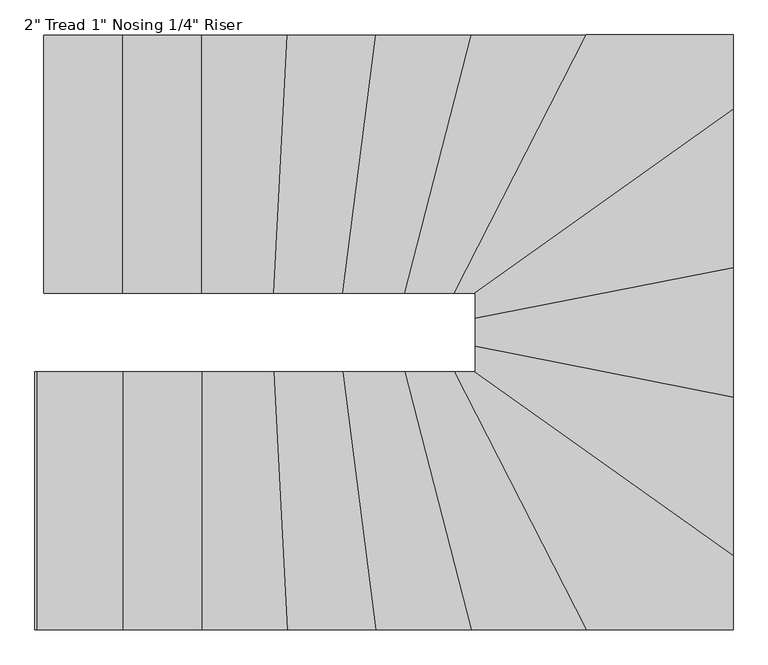
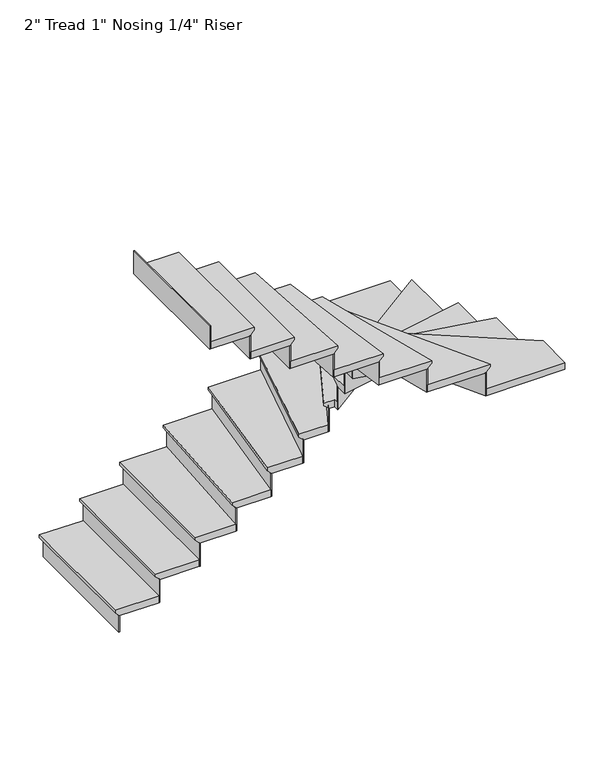
"""IFC4 building model written with IfcOpenShell, lengths in millimetres: stair flight geometry."""

from ifc_helpers import new_model, si_unit, origin, place, context, project, spatial, faceted_brep, source, transform, mapped, element, save


def stair_flight_2bffc1af(model_context):
    return source(origin(), model_context, "Body", "Brep", [
        faceted_brep([(-6984.582258, 1695.3645941, 150.2833333), (-6984.582258, 1695.3645941, 169.3333333), (-6984.582258, 2609.7645941, 169.3333333), (-6984.582258, 2609.7645941, 150.2833333), (-6959.182258, 1695.3645941, 124.8833333), (-6959.182258, 2609.7645941, 124.8833333), (-6679.782258, 1695.3645941, 169.3333333), (-6679.782258, 2609.7645941, 169.3333333), (-6959.182258, 2609.7645941, 118.5333333), (-6679.782258, 2609.7645941, 118.5333333), (-6679.782258, 1695.3645941, 118.5333333), (-6959.182258, 1695.3645941, 118.5333333)], [[[0, 1, 2, 3]], [[4, 0, 3, 5]], [[2, 1, 6, 7]], [[8, 9, 10, 11]], [[2, 7, 9, 8, 5, 3]], [[8, 11, 4, 5]], [[6, 1, 0, 4, 11, 10]], [[7, 6, 10, 9]]]),
        faceted_brep([(-6959.182258, 1695.3645941, 118.5333333), (-6959.182258, 1695.3645941, 0.0), (-6952.832258, 1695.3645941, 0.0), (-6952.832258, 1695.3645941, 118.5333333), (-6959.182258, 2609.7645941, 118.5333333), (-6952.832258, 2609.7645941, 118.5333333), (-6952.832258, 2609.7645941, 0.0), (-6959.182258, 2609.7645941, 0.0)], [[[0, 1, 2, 3]], [[4, 5, 6, 7]], [[1, 0, 4, 7]], [[2, 1, 7, 6]], [[3, 2, 6, 5]], [[0, 3, 5, 4]]]),
        faceted_brep([(-6679.782258, 1695.3645941, 287.8666667), (-6679.782258, 1695.3645941, 118.5333333), (-6673.432258, 1695.3645941, 118.5333333), (-6673.432258, 1695.3645941, 287.8666667), (-6679.782258, 2609.7645941, 287.8666667), (-6673.432258, 2609.7645941, 287.8666667), (-6673.432258, 2609.7645941, 118.5333333), (-6679.782258, 2609.7645941, 118.5333333)], [[[0, 1, 2, 3]], [[4, 5, 6, 7]], [[1, 0, 4, 7]], [[2, 1, 7, 6]], [[3, 2, 6, 5]], [[0, 3, 5, 4]]]),
        faceted_brep([(-6705.182258, 2609.7645941, 338.6666667), (-6705.182258, 1695.3645941, 338.6666667), (-6400.382258, 1695.3645941, 338.6666667), (-6400.382258, 2609.7645941, 338.6666667), (-6679.782258, 2609.7645941, 287.8666667), (-6400.382258, 2609.7645941, 287.8666667), (-6400.382258, 1695.3645941, 287.8666667), (-6679.782258, 1695.3645941, 287.8666667), (-6679.782258, 2609.7645941, 294.2166667), (-6705.182258, 2609.7645941, 319.6166667), (-6679.782258, 1695.3645941, 294.2166667), (-6705.182258, 1695.3645941, 319.6166667)], [[[0, 1, 2, 3]], [[4, 5, 6, 7]], [[0, 3, 5, 4, 8, 9]], [[4, 7, 10, 8]], [[2, 1, 11, 10, 7, 6]], [[3, 2, 6, 5]], [[11, 1, 0, 9]], [[10, 11, 9, 8]]]),
        faceted_brep([(-6400.382258, 1695.3645941, 457.2), (-6400.382258, 1695.3645941, 287.8666667), (-6394.032258, 1695.3645941, 287.8666667), (-6394.032258, 1695.3645941, 457.2), (-6400.382258, 2609.7645941, 457.2), (-6394.032258, 2609.7645941, 457.2), (-6394.032258, 2609.7645941, 287.8666667), (-6400.382258, 2609.7645941, 287.8666667)], [[[0, 1, 2, 3]], [[4, 5, 6, 7]], [[1, 0, 4, 7]], [[2, 1, 7, 6]], [[3, 2, 6, 5]], [[0, 3, 5, 4]]]),
        faceted_brep([(-6425.782258, 2609.7645941, 508.0), (-6425.782258, 1695.3645941, 508.0), (-6144.7150966, 1695.3645941, 508.0), (-6097.1808262, 2609.7645941, 508.0), (-6400.382258, 2609.7645941, 457.2), (-6097.1808262, 2609.7645941, 457.2), (-6144.7150966, 1695.3645941, 457.2), (-6400.382258, 1695.3645941, 457.2), (-6400.382258, 2609.7645941, 463.55), (-6425.782258, 2609.7645941, 488.95), (-6400.382258, 1695.3645941, 463.55), (-6425.782258, 1695.3645941, 488.95)], [[[0, 1, 2, 3]], [[4, 5, 6, 7]], [[0, 3, 5, 4, 8, 9]], [[4, 7, 10, 8]], [[2, 1, 11, 10, 7, 6]], [[3, 2, 6, 5]], [[11, 1, 0, 9]], [[10, 11, 9, 8]]]),
        faceted_brep([(-6144.7150966, 1695.3645941, 626.5333333), (-6144.7150966, 1695.3645941, 457.2), (-6138.3565224, 1695.3645941, 457.2), (-6138.3565224, 1695.3645941, 626.5333333), (-6097.1808262, 2609.7645941, 626.5333333), (-6090.822252, 2609.7645941, 626.5333333), (-6090.822252, 2609.7645941, 457.2), (-6097.1808262, 2609.7645941, 457.2)], [[[0, 1, 2, 3]], [[4, 5, 6, 7]], [[1, 0, 4, 7]], [[2, 1, 7, 6]], [[3, 2, 6, 5]], [[0, 3, 5, 4]]]),
        faceted_brep([(-6122.6151228, 2609.7645941, 677.3333333), (-6170.1493932, 1695.3645941, 677.3333333), (-5900.5483967, 1695.3645941, 677.3333333), (-5782.1923451, 2609.7645941, 677.3333333), (-6097.1808262, 2609.7645941, 626.5333333), (-5782.1923451, 2609.7645941, 626.5333333), (-5900.5483967, 1695.3645941, 626.5333333), (-6144.7150966, 1695.3645941, 626.5333333), (-6097.1808262, 2609.7645941, 632.8833333), (-6122.6151228, 2609.7645941, 658.2833333), (-6144.7150966, 1695.3645941, 632.8833333), (-6170.1493932, 1695.3645941, 658.2833333)], [[[0, 1, 2, 3]], [[4, 5, 6, 7]], [[0, 3, 5, 4, 8, 9]], [[4, 7, 10, 8]], [[2, 1, 11, 10, 7, 6]], [[3, 2, 6, 5]], [[11, 1, 0, 9]], [[10, 11, 9, 8]]]),
        faceted_brep([(-5900.5483967, 1695.3645941, 795.8666667), (-5900.5483967, 1695.3645941, 626.5333333), (-5894.145425, 1695.3645941, 626.5333333), (-5894.145425, 1695.3645941, 795.8666667), (-5782.1923451, 2609.7645941, 795.8666667), (-5775.7893733, 2609.7645941, 795.8666667), (-5775.7893733, 2609.7645941, 626.5333333), (-5782.1923451, 2609.7645941, 626.5333333)], [[[0, 1, 2, 3]], [[4, 5, 6, 7]], [[1, 0, 4, 7]], [[2, 1, 7, 6]], [[3, 2, 6, 5]], [[0, 3, 5, 4]]]),
        faceted_brep([(-5807.8042322, 2609.7645941, 846.6666667), (-5926.1602839, 1695.3645941, 846.6666667), (-5678.9211743, 1695.3645941, 846.6666667), (-5443.7907269, 2609.7645941, 846.6666667), (-5782.1923451, 2609.7645941, 795.8666667), (-5443.7907269, 2609.7645941, 795.8666667), (-5678.9211743, 1695.3645941, 795.8666667), (-5900.5483967, 1695.3645941, 795.8666667), (-5782.1923451, 2609.7645941, 802.2166667), (-5807.8042322, 2609.7645941, 827.6166667), (-5900.5483967, 1695.3645941, 802.2166667), (-5926.1602839, 1695.3645941, 827.6166667)], [[[0, 1, 2, 3]], [[4, 5, 6, 7]], [[0, 3, 5, 4, 8, 9]], [[4, 7, 10, 8]], [[2, 1, 11, 10, 7, 6]], [[3, 2, 6, 5]], [[11, 1, 0, 9]], [[10, 11, 9, 8]]]),
        faceted_brep([(-5678.9211743, 1695.3645941, 965.2), (-5678.9211743, 1695.3645941, 795.8666667), (-5672.3645974, 1695.3645941, 795.8666667), (-5672.3645974, 1695.3645941, 965.2), (-5443.7907269, 2609.7645941, 965.2), (-5437.23415, 2609.7645941, 965.2), (-5437.23415, 2609.7645941, 795.8666667), (-5443.7907269, 2609.7645941, 795.8666667)], [[[0, 1, 2, 3]], [[4, 5, 6, 7]], [[1, 0, 4, 7]], [[2, 1, 7, 6]], [[3, 2, 6, 5]], [[0, 3, 5, 4]]]),
        faceted_brep([(-5470.0170343, 2609.7645941, 1016.0), (-5705.1474817, 1695.3645941, 1016.0), (-5502.5745382, 1695.3645941, 1016.0), (-5033.7499169, 2609.7645941, 1016.0), (-5443.7907269, 2609.7645941, 965.2), (-5033.7499169, 2609.7645941, 965.2), (-5502.5745382, 1695.3645941, 965.2), (-5678.9211743, 1695.3645941, 965.2), (-5443.7907269, 2609.7645941, 971.55), (-5470.0170343, 2609.7645941, 996.95), (-5678.9211743, 1695.3645941, 971.55), (-5705.1474817, 1695.3645941, 996.95)], [[[0, 1, 2, 3]], [[4, 5, 6, 7]], [[0, 3, 5, 4, 8, 9]], [[4, 7, 10, 8]], [[2, 1, 11, 10, 7, 6]], [[3, 2, 6, 5]], [[11, 1, 0, 9]], [[10, 11, 9, 8]]]),
        faceted_brep([(-5502.5745382, 1695.3645941, 1134.5333333), (-5502.5745382, 1695.3645941, 965.2), (-5495.4385551, 1695.3645941, 965.2), (-5495.4385551, 1695.3645941, 1134.5333333), (-5033.7499169, 2609.7645941, 1134.5333333), (-5026.6139337, 2609.7645941, 1134.5333333), (-5026.6139337, 2609.7645941, 965.2), (-5033.7499169, 2609.7645941, 965.2)], [[[0, 1, 2, 3]], [[4, 5, 6, 7]], [[1, 0, 4, 7]], [[2, 1, 7, 6]], [[3, 2, 6, 5]], [[0, 3, 5, 4]]]),
        faceted_brep([(-4542.4505662, 2316.0834604, 1185.3333333), (-4542.4505662, 2609.7645941, 1185.3333333), (-5062.2938494, 2609.7645941, 1185.3333333), (-5531.1184707, 1695.3645941, 1185.3333333), (-5456.8505662, 1695.3645941, 1185.3333333), (-5456.8505662, 1665.8095113, 1185.3333333), (-4542.4505662, 2609.7645941, 1134.5333333), (-4542.4505662, 2316.0834604, 1134.5333333), (-5456.8505662, 1665.8095113, 1134.5333333), (-5456.8505662, 1695.3645941, 1134.5333333), (-5502.5745382, 1695.3645941, 1134.5333333), (-5033.7499169, 2609.7645941, 1134.5333333), (-5033.7499169, 2609.7645941, 1140.8833333), (-5062.2938494, 2609.7645941, 1166.2833333), (-5502.5745382, 1695.3645941, 1140.8833333), (-5531.1184707, 1695.3645941, 1166.2833333)], [[[0, 1, 2, 3, 4, 5]], [[6, 7, 8, 9, 10, 11]], [[1, 0, 7, 6]], [[2, 1, 6, 11, 12, 13]], [[11, 10, 14, 12]], [[4, 3, 15, 14, 10, 9]], [[5, 4, 9, 8]], [[0, 5, 8, 7]], [[15, 3, 2, 13]], [[14, 15, 13, 12]]]),
        faceted_brep([(-5456.8505662, 1665.8095113, 1303.8666667), (-5456.8505662, 1665.8095113, 1134.5333333), (-5456.8505662, 1658.0175365, 1134.5333333), (-5456.8505662, 1658.0175365, 1303.8666667), (-4542.4505662, 2316.0834604, 1303.8666667), (-4542.4505662, 2308.2914857, 1303.8666667), (-4542.4505662, 2308.2914857, 1134.5333333), (-4542.4505662, 2316.0834604, 1134.5333333)], [[[0, 1, 2, 3]], [[4, 5, 6, 7]], [[1, 0, 4, 7]], [[2, 1, 7, 6]], [[3, 2, 6, 5]], [[0, 3, 5, 4]]]),
        faceted_brep([(-4542.4505662, 2347.2513596, 1354.6666667), (-5456.8505662, 1696.9774105, 1354.6666667), (-5456.8505662, 1579.3554242, 1354.6666667), (-4542.4505662, 1759.5962806, 1354.6666667), (-4542.4505662, 2316.0834604, 1303.8666667), (-4542.4505662, 1759.5962806, 1303.8666667), (-5456.8505662, 1579.3554242, 1303.8666667), (-5456.8505662, 1665.8095113, 1303.8666667), (-4542.4505662, 2316.0834604, 1310.2166667), (-4542.4505662, 2347.2513596, 1335.6166667), (-5456.8505662, 1665.8095113, 1310.2166667), (-5456.8505662, 1696.9774105, 1335.6166667)], [[[0, 1, 2, 3]], [[4, 5, 6, 7]], [[0, 3, 5, 4, 8, 9]], [[4, 7, 10, 8]], [[2, 1, 11, 10, 7, 6]], [[3, 2, 6, 5]], [[11, 1, 0, 9]], [[10, 11, 9, 8]]]),
        faceted_brep([(-5456.8505662, 1579.3554242, 1473.2), (-5456.8505662, 1579.3554242, 1303.8666667), (-5456.8505662, 1572.8832388, 1303.8666667), (-5456.8505662, 1572.8832388, 1473.2), (-4542.4505662, 1759.5962806, 1473.2), (-4542.4505662, 1753.1240951, 1473.2), (-4542.4505662, 1753.1240951, 1303.8666667), (-4542.4505662, 1759.5962806, 1303.8666667)], [[[0, 1, 2, 3]], [[4, 5, 6, 7]], [[1, 0, 4, 7]], [[2, 1, 7, 6]], [[3, 2, 6, 5]], [[0, 3, 5, 4]]]),
        faceted_brep([(-4542.4505662, 1785.4850223, 1524.0), (-5456.8505662, 1605.244166, 1524.0), (-5456.8505662, 1480.1962806, 1524.0), (-4542.4505662, 1299.9554242, 1524.0), (-4542.4505662, 1759.5962806, 1473.2), (-4542.4505662, 1299.9554242, 1473.2), (-5456.8505662, 1480.1962806, 1473.2), (-5456.8505662, 1579.3554242, 1473.2), (-4542.4505662, 1759.5962806, 1479.55), (-4542.4505662, 1785.4850223, 1504.95), (-5456.8505662, 1579.3554242, 1479.55), (-5456.8505662, 1605.244166, 1504.95)], [[[0, 1, 2, 3]], [[4, 5, 6, 7]], [[0, 3, 5, 4, 8, 9]], [[4, 7, 10, 8]], [[2, 1, 11, 10, 7, 6]], [[3, 2, 6, 5]], [[11, 1, 0, 9]], [[10, 11, 9, 8]]]),
        faceted_brep([(-5456.8505662, 1480.1962806, 1642.5333333), (-5456.8505662, 1480.1962806, 1473.2), (-5456.8505662, 1473.7240951, 1473.2), (-5456.8505662, 1473.7240951, 1642.5333333), (-4542.4505662, 1299.9554242, 1642.5333333), (-4542.4505662, 1293.4832388, 1642.5333333), (-4542.4505662, 1293.4832388, 1473.2), (-4542.4505662, 1299.9554242, 1473.2)], [[[0, 1, 2, 3]], [[4, 5, 6, 7]], [[1, 0, 4, 7]], [[2, 1, 7, 6]], [[3, 2, 6, 5]], [[0, 3, 5, 4]]]),
        faceted_brep([(-4542.4505662, 1325.844166, 1693.3333333), (-5456.8505662, 1506.0850223, 1693.3333333), (-5456.8505662, 1415.9645941, 1693.3333333), (-5502.9460407, 1415.9645941, 1693.3333333), (-4542.4505662, 732.9099295, 1693.3333333), (-4542.4505662, 1299.9554242, 1642.5333333), (-4542.4505662, 732.9099295, 1642.5333333), (-5502.9460407, 1415.9645941, 1642.5333333), (-5456.8505662, 1415.9645941, 1642.5333333), (-5456.8505662, 1480.1962806, 1642.5333333), (-4542.4505662, 1299.9554242, 1648.8833333), (-4542.4505662, 1325.844166, 1674.2833333), (-5456.8505662, 1480.1962806, 1648.8833333), (-5456.8505662, 1506.0850223, 1674.2833333)], [[[0, 1, 2, 3, 4]], [[5, 6, 7, 8, 9]], [[0, 4, 6, 5, 10, 11]], [[5, 9, 12, 10]], [[2, 1, 13, 12, 9, 8]], [[3, 2, 8, 7]], [[4, 3, 7, 6]], [[13, 1, 0, 11]], [[12, 13, 11, 10]]]),
        faceted_brep([(-5502.9460407, 1415.9645941, 1811.8666667), (-5502.9460407, 1415.9645941, 1642.5333333), (-5513.9029332, 1415.9645941, 1642.5333333), (-5513.9029332, 1415.9645941, 1811.8666667), (-4542.4505662, 732.9099295, 1811.8666667), (-4542.4505662, 725.1179547, 1811.8666667), (-4542.4505662, 725.1179547, 1642.5333333), (-4542.4505662, 732.9099295, 1642.5333333)], [[[0, 1, 2, 3]], [[4, 5, 6, 7]], [[1, 0, 4, 7]], [[2, 1, 7, 6]], [[3, 2, 6, 5]], [[0, 3, 5, 4]]]),
        faceted_brep([(-5090.8377819, 501.5645941, 1862.6666667), (-4542.4505662, 501.5645941, 1862.6666667), (-4542.4505662, 764.0778287, 1862.6666667), (-5459.1184707, 1415.9645941, 1862.6666667), (-5559.6624033, 1415.9645941, 1862.6666667), (-4542.4505662, 501.5645941, 1811.8666667), (-5090.8377819, 501.5645941, 1811.8666667), (-5559.6624033, 1415.9645941, 1811.8666667), (-5502.9460407, 1415.9645941, 1811.8666667), (-4542.4505662, 732.9099295, 1811.8666667), (-4542.4505662, 732.9099295, 1818.2166667), (-4542.4505662, 764.0778287, 1843.6166667), (-5502.9460407, 1415.9645941, 1818.2166667), (-5459.1184707, 1415.9645941, 1843.6166667)], [[[0, 1, 2, 3, 4]], [[5, 6, 7, 8, 9]], [[1, 0, 6, 5]], [[2, 1, 5, 9, 10, 11]], [[9, 8, 12, 10]], [[4, 3, 13, 12, 8, 7]], [[0, 4, 7, 6]], [[13, 3, 2, 11]], [[12, 13, 11, 10]]]),
        faceted_brep([(-5559.6624033, 1415.9645941, 1981.2), (-5559.6624033, 1415.9645941, 1811.8666667), (-5566.7983864, 1415.9645941, 1811.8666667), (-5566.7983864, 1415.9645941, 1981.2), (-5090.8377819, 501.5645941, 1981.2), (-5097.9737651, 501.5645941, 1981.2), (-5097.9737651, 501.5645941, 1811.8666667), (-5090.8377819, 501.5645941, 1811.8666667)], [[[0, 1, 2, 3]], [[4, 5, 6, 7]], [[1, 0, 4, 7]], [[2, 1, 7, 6]], [[3, 2, 6, 5]], [[0, 3, 5, 4]]]),
        faceted_brep([(-5062.2938494, 501.5645941, 2032.0), (-5531.1184707, 1415.9645941, 2032.0), (-5731.3737892, 1415.9645941, 2032.0), (-5496.2433418, 501.5645941, 2032.0), (-5090.8377819, 501.5645941, 1981.2), (-5496.2433418, 501.5645941, 1981.2), (-5731.3737892, 1415.9645941, 1981.2), (-5559.6624033, 1415.9645941, 1981.2), (-5090.8377819, 501.5645941, 1987.55), (-5062.2938494, 501.5645941, 2012.95), (-5559.6624033, 1415.9645941, 1987.55), (-5531.1184707, 1415.9645941, 2012.95)], [[[0, 1, 2, 3]], [[4, 5, 6, 7]], [[0, 3, 5, 4, 8, 9]], [[4, 7, 10, 8]], [[2, 1, 11, 10, 7, 6]], [[3, 2, 6, 5]], [[11, 1, 0, 9]], [[10, 11, 9, 8]]]),
        faceted_brep([(-5731.3737892, 1415.9645941, 2150.5333333), (-5731.3737892, 1415.9645941, 1981.2), (-5737.9303661, 1415.9645941, 1981.2), (-5737.9303661, 1415.9645941, 2150.5333333), (-5496.2433418, 501.5645941, 2150.5333333), (-5502.7999187, 501.5645941, 2150.5333333), (-5502.7999187, 501.5645941, 1981.2), (-5496.2433418, 501.5645941, 1981.2)], [[[0, 1, 2, 3]], [[4, 5, 6, 7]], [[1, 0, 4, 7]], [[2, 1, 7, 6]], [[3, 2, 6, 5]], [[0, 3, 5, 4]]]),
        faceted_brep([(-5470.0170343, 501.5645941, 2201.3333333), (-5705.1474817, 1415.9645941, 2201.3333333), (-5951.772171, 1415.9645941, 2201.3333333), (-5833.4161193, 501.5645941, 2201.3333333), (-5496.2433418, 501.5645941, 2150.5333333), (-5833.4161193, 501.5645941, 2150.5333333), (-5951.772171, 1415.9645941, 2150.5333333), (-5731.3737892, 1415.9645941, 2150.5333333), (-5496.2433418, 501.5645941, 2156.8833333), (-5470.0170343, 501.5645941, 2182.2833333), (-5731.3737892, 1415.9645941, 2156.8833333), (-5705.1474817, 1415.9645941, 2182.2833333)], [[[0, 1, 2, 3]], [[4, 5, 6, 7]], [[0, 3, 5, 4, 8, 9]], [[4, 7, 10, 8]], [[2, 1, 11, 10, 7, 6]], [[3, 2, 6, 5]], [[11, 1, 0, 9]], [[10, 11, 9, 8]]]),
        faceted_brep([(-5951.772171, 1415.9645941, 2319.8666667), (-5951.772171, 1415.9645941, 2150.5333333), (-5958.1751428, 1415.9645941, 2150.5333333), (-5958.1751428, 1415.9645941, 2319.8666667), (-5833.4161193, 501.5645941, 2319.8666667), (-5839.8190911, 501.5645941, 2319.8666667), (-5839.8190911, 501.5645941, 2150.5333333), (-5833.4161193, 501.5645941, 2150.5333333)], [[[0, 1, 2, 3]], [[4, 5, 6, 7]], [[1, 0, 4, 7]], [[2, 1, 7, 6]], [[3, 2, 6, 5]], [[0, 3, 5, 4]]]),
        faceted_brep([(-5807.8042322, 501.5645941, 2370.6666667), (-5926.1602839, 1415.9645941, 2370.6666667), (-6195.5836899, 1415.9645941, 2370.6666667), (-6148.0494195, 501.5645941, 2370.6666667), (-5833.4161193, 501.5645941, 2319.8666667), (-6148.0494195, 501.5645941, 2319.8666667), (-6195.5836899, 1415.9645941, 2319.8666667), (-5951.772171, 1415.9645941, 2319.8666667), (-5833.4161193, 501.5645941, 2326.2166667), (-5807.8042322, 501.5645941, 2351.6166667), (-5951.772171, 1415.9645941, 2326.2166667), (-5926.1602839, 1415.9645941, 2351.6166667)], [[[0, 1, 2, 3]], [[4, 5, 6, 7]], [[0, 3, 5, 4, 8, 9]], [[4, 7, 10, 8]], [[2, 1, 11, 10, 7, 6]], [[3, 2, 6, 5]], [[11, 1, 0, 9]], [[10, 11, 9, 8]]]),
        faceted_brep([(-6195.5836899, 1415.9645941, 2489.2), (-6195.5836899, 1415.9645941, 2319.8666667), (-6201.9422641, 1415.9645941, 2319.8666667), (-6201.9422641, 1415.9645941, 2489.2), (-6148.0494195, 501.5645941, 2489.2), (-6154.4079937, 501.5645941, 2489.2), (-6154.4079937, 501.5645941, 2319.8666667), (-6148.0494195, 501.5645941, 2319.8666667)], [[[0, 1, 2, 3]], [[4, 5, 6, 7]], [[1, 0, 4, 7]], [[2, 1, 7, 6]], [[3, 2, 6, 5]], [[0, 3, 5, 4]]]),
        faceted_brep([(-6122.6151228, 501.5645941, 2540.0), (-6170.1493932, 1415.9645941, 2540.0), (-6451.182258, 1415.9645941, 2540.0), (-6451.182258, 501.5645941, 2540.0), (-6148.0494195, 501.5645941, 2489.2), (-6451.182258, 501.5645941, 2489.2), (-6451.182258, 1415.9645941, 2489.2), (-6195.5836899, 1415.9645941, 2489.2), (-6148.0494195, 501.5645941, 2495.55), (-6122.6151228, 501.5645941, 2520.95), (-6195.5836899, 1415.9645941, 2495.55), (-6170.1493932, 1415.9645941, 2520.95)], [[[0, 1, 2, 3]], [[4, 5, 6, 7]], [[0, 3, 5, 4, 8, 9]], [[4, 7, 10, 8]], [[2, 1, 11, 10, 7, 6]], [[3, 2, 6, 5]], [[11, 1, 0, 9]], [[10, 11, 9, 8]]]),
        faceted_brep([(-6451.182258, 1415.9645941, 2658.5333333), (-6451.182258, 1415.9645941, 2489.2), (-6457.532258, 1415.9645941, 2489.2), (-6457.532258, 1415.9645941, 2658.5333333), (-6451.182258, 501.5645941, 2658.5333333), (-6457.532258, 501.5645941, 2658.5333333), (-6457.532258, 501.5645941, 2489.2), (-6451.182258, 501.5645941, 2489.2)], [[[0, 1, 2, 3]], [[4, 5, 6, 7]], [[1, 0, 4, 7]], [[2, 1, 7, 6]], [[3, 2, 6, 5]], [[0, 3, 5, 4]]]),
        faceted_brep([(-6425.782258, 501.5645941, 2709.3333333), (-6425.782258, 1415.9645941, 2709.3333333), (-6730.582258, 1415.9645941, 2709.3333333), (-6730.582258, 501.5645941, 2709.3333333), (-6451.182258, 501.5645941, 2658.5333333), (-6730.582258, 501.5645941, 2658.5333333), (-6730.582258, 1415.9645941, 2658.5333333), (-6451.182258, 1415.9645941, 2658.5333333), (-6451.182258, 501.5645941, 2664.8833333), (-6425.782258, 501.5645941, 2690.2833333), (-6451.182258, 1415.9645941, 2664.8833333), (-6425.782258, 1415.9645941, 2690.2833333)], [[[0, 1, 2, 3]], [[4, 5, 6, 7]], [[0, 3, 5, 4, 8, 9]], [[4, 7, 10, 8]], [[2, 1, 11, 10, 7, 6]], [[3, 2, 6, 5]], [[11, 1, 0, 9]], [[10, 11, 9, 8]]]),
        faceted_brep([(-6730.582258, 1415.9645941, 2827.8666667), (-6730.582258, 1415.9645941, 2658.5333333), (-6736.932258, 1415.9645941, 2658.5333333), (-6736.932258, 1415.9645941, 2827.8666667), (-6730.582258, 501.5645941, 2827.8666667), (-6736.932258, 501.5645941, 2827.8666667), (-6736.932258, 501.5645941, 2658.5333333), (-6730.582258, 501.5645941, 2658.5333333)], [[[0, 1, 2, 3]], [[4, 5, 6, 7]], [[1, 0, 4, 7]], [[2, 1, 7, 6]], [[3, 2, 6, 5]], [[0, 3, 5, 4]]]),
        faceted_brep([(-7009.982258, 1415.9645941, 2997.2), (-7009.982258, 1415.9645941, 2827.8666667), (-7016.332258, 1415.9645941, 2827.8666667), (-7016.332258, 1415.9645941, 2997.2), (-7009.982258, 501.5645941, 2997.2), (-7016.332258, 501.5645941, 2997.2), (-7016.332258, 501.5645941, 2827.8666667), (-7009.982258, 501.5645941, 2827.8666667)], [[[0, 1, 2, 3]], [[4, 5, 6, 7]], [[1, 0, 4, 7]], [[2, 1, 7, 6]], [[3, 2, 6, 5]], [[0, 3, 5, 4]]]),
        faceted_brep([(-6705.182258, 501.5645941, 2878.6666667), (-6705.182258, 1415.9645941, 2878.6666667), (-7009.982258, 1415.9645941, 2878.6666667), (-7009.982258, 501.5645941, 2878.6666667), (-6730.582258, 501.5645941, 2827.8666667), (-7009.982258, 501.5645941, 2827.8666667), (-7009.982258, 1415.9645941, 2827.8666667), (-6730.582258, 1415.9645941, 2827.8666667), (-6730.582258, 501.5645941, 2834.2166667), (-6705.182258, 501.5645941, 2859.6166667), (-6730.582258, 1415.9645941, 2834.2166667), (-6705.182258, 1415.9645941, 2859.6166667)], [[[0, 1, 2, 3]], [[4, 5, 6, 7]], [[0, 3, 5, 4, 8, 9]], [[4, 7, 10, 8]], [[2, 1, 11, 10, 7, 6]], [[3, 2, 6, 5]], [[11, 1, 0, 9]], [[10, 11, 9, 8]]]),
    ])


if __name__ == "__main__":
    model = new_model("IFC4")
    model_context = context("Model", 3, world=origin())
    ifc_project = project(units=[si_unit("LENGTHUNIT", "METRE", prefix="MILLI")], contexts=[model_context])
    site = spatial("IfcSite", under=ifc_project)
    building = spatial("IfcBuilding", under=site)
    placement = place(None, origin())
    stair_flight_shape = stair_flight_2bffc1af(model_context)
    element("IfcStairFlight", 1, ObjectType="2\" Tread 1\" Nosing 1/4\" Riser", at=placement, inside=building, context=model_context, shape_type="MappedRepresentation", body=[
        mapped(stair_flight_shape, transform((0.0, 0.0, 0.0), x_axis=(1.0, 0.0, 0.0), y_axis=(0.0, 1.0, 0.0), z_axis=(0.0, 0.0, 1.0))),
    ])
    save(model, "model.ifc")
